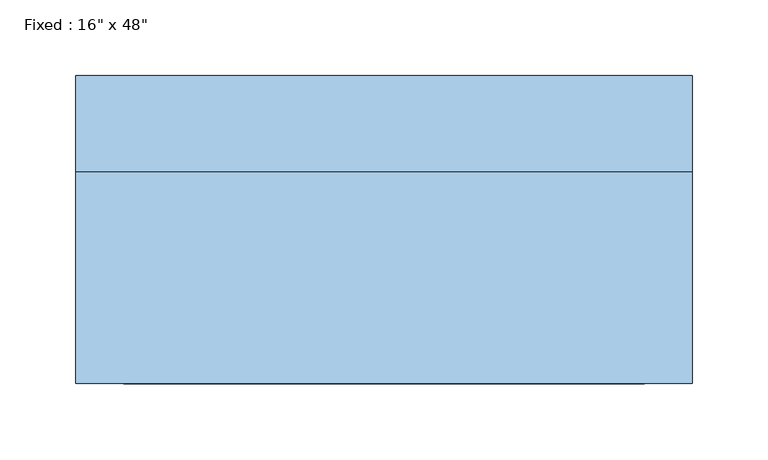
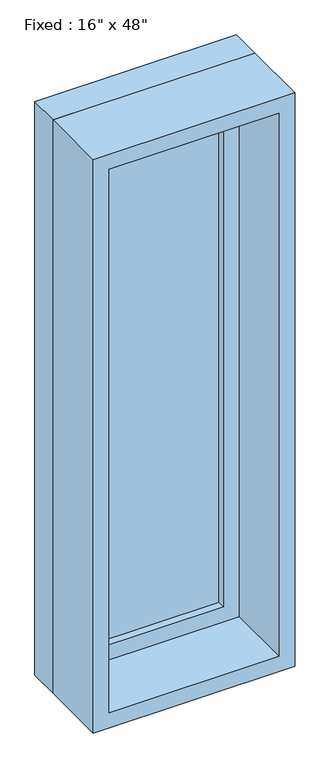
"""IFC4 building model written with IfcOpenShell, lengths in millimetres: window geometry."""

from ifc_helpers import new_model, si_unit, frame, origin, place, context, project, spatial, polyline, outline, extrude, source, transform, mapped, element, save


def window_f81341e8(model_context):
    return source(origin(), model_context, "Body", "SweptSolid", [
        extrude(outline(polyline([(101.6, 53.975), (-177.8, 53.975), (-177.8, 66.675), (101.6, 66.675), (101.6, 53.975)])), frame((0.0, 0.0, 977.9), z_axis=(0.0, 0.0, 1.0), x_axis=(1.0, 0.0, 0.0)), (0.0, 0.0, 1.0), 1092.2),
        extrude(outline(polyline([(2114.55, -222.25), (933.45, -222.25), (933.45, 146.05), (2114.55, 146.05), (2114.55, -222.25)]), holes=[polyline([(2070.1, -177.8), (2070.1, 101.6), (977.9, 101.6), (977.9, -177.8), (2070.1, -177.8)])]), frame((0.0, 38.1, 0.0), z_axis=(0.0, 1.0, 0.0), x_axis=(0.0, 0.0, 1.0)), (0.0, 0.0, 1.0), 44.45),
        extrude(outline(polyline([(2133.6, -241.3), (914.4, -241.3), (914.4, 165.1), (2133.6, 165.1), (2133.6, -241.3)]), holes=[polyline([(2101.85, -209.55), (2101.85, 133.35), (946.15, 133.35), (946.15, -209.55), (2101.85, -209.55)])]), frame((0.0, -101.6, 0.0), z_axis=(0.0, 1.0, 0.0), x_axis=(0.0, 0.0, 1.0)), (0.0, 0.0, 1.0), 139.7),
        extrude(outline(polyline([(2133.6, 165.1), (2133.6, -241.3), (914.4, -241.3), (914.4, 165.1), (2133.6, 165.1)]), holes=[polyline([(2114.55, 146.05), (933.45, 146.05), (933.45, -222.25), (2114.55, -222.25), (2114.55, 146.05)])]), frame((0.0, 38.1, 0.0), z_axis=(0.0, 1.0, 0.0), x_axis=(0.0, 0.0, 1.0)), (0.0, 0.0, 1.0), 63.5),
    ])


if __name__ == "__main__":
    model = new_model("IFC4")
    model_context = context("Model", 3, world=origin())
    ifc_project = project(units=[si_unit("LENGTHUNIT", "METRE", prefix="MILLI")], contexts=[model_context])
    site = spatial("IfcSite", under=ifc_project)
    building = spatial("IfcBuilding", under=site)
    placement = place(None, origin())
    window_shape = window_f81341e8(model_context)
    element("IfcWindow", 1, ObjectType="Fixed : 16\" x 48\"", at=placement, inside=building, context=model_context, shape_type="MappedRepresentation", body=[
        mapped(window_shape, transform((0.0, 0.0, 0.0), x_axis=(1.0, 0.0, 0.0), y_axis=(0.0, 1.0, 0.0), z_axis=(0.0, 0.0, 1.0))),
    ])
    save(model, "model.ifc")

# Revit data of these elements
# Type "Fixed : 16\" x 48\""
#   Type Mark = "5"
#   Construction Type Id = "GSP4R"
#   Assembly Code = "B2020100"
#   Analytic Construction = "1/8 in Pilkington single glazing"
#   Visual Light Transmittance = 0.9
#   Solar Heat Gain Coefficient = 0.78
#   Heat Transfer Coefficient (U) = 0.6496 BTU/(h·ft²·°F)
#   Height = 4' - 0"
#   Default Sill Height = 3' - 0"
#   Width = 1' - 4"
#   Window Inset = 0' - 0 3/4"
#   Define Thermal Properties by = 1
#   Glass Pane Material = Glass
#   Sash Material = Sash
#   Wall Closure = (empty or 0)
# Element 1 (IfcWindow, "Fixed : 16\" x 48\"")
#   Materials on its faces: "Sash", "Glass"
# Materials
#   "Glass": class "Glass", colour RGB 0 128 192, transparency 0.75, Description = "Soda Lime Glass", Cost = 0
#   "Sash": class "Wood", colour RGB 224 178 126, transparency 0
